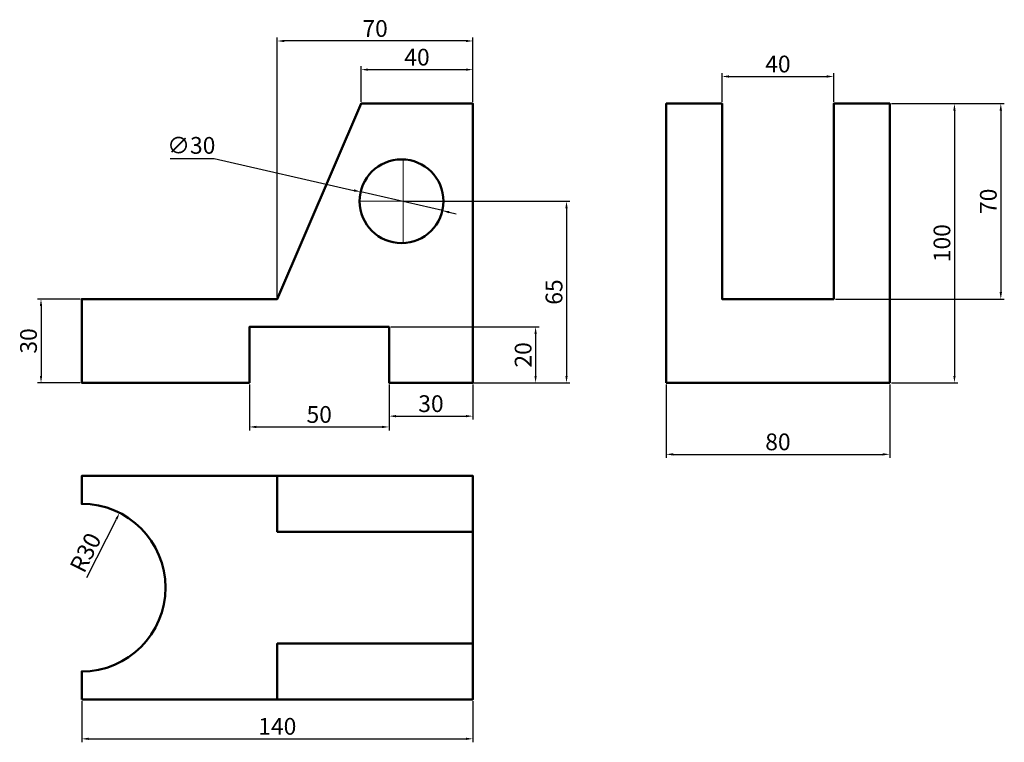
# Model space of a CAD drawing. Units: millimetres. Extents: x 2 to 354, y 5 to 263.
import ezdxf

# ---------------------------------------------------------------- set-up
doc = ezdxf.new("R2010")
doc.units = ezdxf.units.MM
doc.linetypes.add('CENTER', pattern=[50.8, 31.75, -6.35, 6.35, -6.35])
for name, color, linetype, lineweight in [('M-CNTR', 1, 'CENTER', 18), ('M-DIMS', 2, 'Continuous', 25), ('M-OUTL', 7, 'Continuous', 50)]:
    doc.layers.add(name, color=color, linetype=linetype, lineweight=lineweight)
doc.styles.get("Standard").update_dxf_attribs({"font": 'arial.ttf'})
doc.dimstyles.new('ISO-25', dxfattribs={"dimtxt": 6, "dimasz": 2.5, "dimexe": 1.25, "dimexo": 0.625, "dimtad": 1, "dimtoh": 1, "dimdec": 0, "dimtxsty": 'Standard', "dimcen": 2.5, "dimadec": 0, "dimazin": 0, "dimtfac": 1, "dimtdec": 0, "dimtmove": 0, "dimatfit": 3, "dimfxl": 1, "dimarcsym": 0})

# ---------------------------------------------------------------- blocks, each defined once
blk = doc.blocks.new('*D1')
at = {"layer": 'Defpoints', "color": 0, "transparency": 16777216}
for p in [(93.8, 255.73), (163.8, 233.33), (93.8, 163.33)]:
    blk.add_point(p, dxfattribs=at)
at = {"layer": 'M-DIMS', "color": 0, "lineweight": -2, "transparency": 16777216}
for p, q in [((93.8, 163.96), (93.8, 256.98)), ((161.3, 255.73), (96.3, 255.73)), ((163.8, 233.96), (163.8, 256.98))]:
    blk.add_line(p, q, dxfattribs=at)
at = {"layer": 'M-DIMS', "color": 0, "transparency": 16777216}
for points in [[(96.3, 256.14), (96.3, 255.31), (93.8, 255.73)], [(161.3, 256.14), (161.3, 255.31), (163.8, 255.73)]]:
    blk.add_solid(points, dxfattribs=at)
at = {"layer": 'M-DIMS', "color": 0, "transparency": 16777216, "insert": (128.8, 259.42), "char_height": 6, "attachment_point": 5}
blk.add_mtext('70', dxfattribs=at)
blk = doc.blocks.new('*D2')
at = {"layer": 'Defpoints', "color": 0, "transparency": 16777216}
for p in [(163.8, 245.47), (123.8, 233.33), (163.8, 233.33)]:
    blk.add_point(p, dxfattribs=at)
at = {"layer": 'M-DIMS', "color": 0, "lineweight": -2, "transparency": 16777216}
for p, q in [((123.8, 233.96), (123.8, 246.72)), ((163.8, 233.96), (163.8, 246.72)), ((126.3, 245.47), (161.3, 245.47))]:
    blk.add_line(p, q, dxfattribs=at)
at = {"layer": 'M-DIMS', "color": 0, "transparency": 16777216}
for points in [[(126.3, 245.88), (126.3, 245.05), (123.8, 245.47)], [(161.3, 245.88), (161.3, 245.05), (163.8, 245.47)]]:
    blk.add_solid(points, dxfattribs=at)
at = {"layer": 'M-DIMS', "color": 0, "transparency": 16777216, "insert": (143.8, 249.16), "char_height": 6, "attachment_point": 5}
blk.add_mtext('40', dxfattribs=at)
blk = doc.blocks.new('*D3')
at = {"layer": 'Defpoints', "color": 0, "transparency": 16777216}
for p in [(133.8, 153.33), (133.8, 133.33), (186.25, 133.33)]:
    blk.add_point(p, dxfattribs=at)
at = {"layer": 'M-DIMS', "color": 0, "lineweight": -2, "transparency": 16777216}
for p, q in [((134.43, 153.33), (187.5, 153.33)), ((186.25, 150.83), (186.25, 135.83)), ((134.43, 133.33), (187.5, 133.33))]:
    blk.add_line(p, q, dxfattribs=at)
at = {"layer": 'M-DIMS', "color": 0, "transparency": 16777216}
for points in [[(185.84, 150.83), (186.67, 150.83), (186.25, 153.33)], [(185.84, 135.83), (186.67, 135.83), (186.25, 133.33)]]:
    blk.add_solid(points, dxfattribs=at)
at = {"layer": 'M-DIMS', "color": 0, "transparency": 16777216, "insert": (182.57, 143.33), "char_height": 6, "attachment_point": 5, "rotation": 90}
blk.add_mtext('20', dxfattribs=at)
blk = doc.blocks.new('*D4')
at = {"layer": 'Defpoints', "color": 0, "transparency": 16777216}
for p in [(138.8, 198.33), (133.8, 133.33), (197.32, 133.33)]:
    blk.add_point(p, dxfattribs=at)
at = {"layer": 'M-DIMS', "color": 0, "lineweight": -2, "transparency": 16777216}
for p, q in [((139.43, 198.33), (198.57, 198.33)), ((197.32, 195.83), (197.32, 135.83)), ((134.43, 133.33), (198.57, 133.33))]:
    blk.add_line(p, q, dxfattribs=at)
at = {"layer": 'M-DIMS', "color": 0, "transparency": 16777216}
for points in [[(196.9, 195.83), (197.74, 195.83), (197.32, 198.33)], [(196.9, 135.83), (197.74, 135.83), (197.32, 133.33)]]:
    blk.add_solid(points, dxfattribs=at)
at = {"layer": 'M-DIMS', "color": 0, "transparency": 16777216, "insert": (193.63, 165.83), "char_height": 6, "attachment_point": 5, "rotation": 90}
blk.add_mtext('65', dxfattribs=at)
blk = doc.blocks.new('*D5')
at = {"layer": 'Defpoints', "color": 0, "transparency": 16777216}
for p in [(123.66, 201.68), (152.9, 194.98)]:
    blk.add_point(p, dxfattribs=at)
at = {"layer": 'M-DIMS', "color": 0, "lineweight": -2, "transparency": 16777216}
for p, q in [((55.45, 213.71), (71.18, 213.71)), ((71.18, 213.71), (121.22, 202.24)), ((152.9, 194.98), (123.66, 201.68)), ((155.34, 194.42), (157.77, 193.86))]:
    blk.add_line(p, q, dxfattribs=at)
at = {"layer": 'M-DIMS', "color": 0, "transparency": 16777216}
for points in [[(121.31, 202.65), (121.13, 201.84), (123.66, 201.68)], [(155.43, 194.83), (155.24, 194.02), (152.9, 194.98)]]:
    blk.add_solid(points, dxfattribs=at)
at = {"layer": 'M-DIMS', "color": 0, "transparency": 16777216, "insert": (63, 217.57), "char_height": 6, "attachment_point": 5}
blk.add_mtext('∅30', dxfattribs=at)
blk = doc.blocks.new('*D6')
at = {"layer": 'Defpoints', "color": 0, "transparency": 16777216}
for p in [(23.8, 163.33), (9.22, 133.33), (23.8, 133.33)]:
    blk.add_point(p, dxfattribs=at)
at = {"layer": 'M-DIMS', "color": 0, "lineweight": -2, "transparency": 16777216}
for p, q in [((23.18, 163.33), (7.97, 163.33)), ((9.22, 160.83), (9.22, 135.83)), ((23.18, 133.33), (7.97, 133.33))]:
    blk.add_line(p, q, dxfattribs=at)
at = {"layer": 'M-DIMS', "color": 0, "transparency": 16777216}
for points in [[(8.8, 160.83), (9.63, 160.83), (9.22, 163.33)], [(8.8, 135.83), (9.63, 135.83), (9.22, 133.33)]]:
    blk.add_solid(points, dxfattribs=at)
at = {"layer": 'M-DIMS', "color": 0, "transparency": 16777216, "insert": (5.52, 148.33), "char_height": 6, "attachment_point": 5, "rotation": 90}
blk.add_mtext('30', dxfattribs=at)
blk = doc.blocks.new('*D7')
at = {"layer": 'Defpoints', "color": 0, "transparency": 16777216}
for p in [(83.8, 133.33), (133.8, 133.33), (133.8, 117.53)]:
    blk.add_point(p, dxfattribs=at)
at = {"layer": 'M-DIMS', "color": 0, "lineweight": -2, "transparency": 16777216}
for p, q in [((83.8, 132.71), (83.8, 116.28)), ((133.8, 132.71), (133.8, 116.28)), ((86.3, 117.53), (131.3, 117.53))]:
    blk.add_line(p, q, dxfattribs=at)
at = {"layer": 'M-DIMS', "color": 0, "transparency": 16777216}
for points in [[(86.3, 117.95), (86.3, 117.11), (83.8, 117.53)], [(131.3, 117.95), (131.3, 117.11), (133.8, 117.53)]]:
    blk.add_solid(points, dxfattribs=at)
at = {"layer": 'M-DIMS', "color": 0, "transparency": 16777216, "insert": (108.8, 121.22), "char_height": 6, "attachment_point": 5}
blk.add_mtext('50', dxfattribs=at)
blk = doc.blocks.new('*D8')
at = {"layer": 'Defpoints', "color": 0, "transparency": 16777216}
for p in [(133.8, 133.33), (163.8, 133.33), (163.8, 121.4)]:
    blk.add_point(p, dxfattribs=at)
at = {"layer": 'M-DIMS', "color": 0, "lineweight": -2, "transparency": 16777216}
for p, q in [((133.8, 132.71), (133.8, 120.15)), ((163.8, 132.71), (163.8, 120.15)), ((136.3, 121.4), (161.3, 121.4))]:
    blk.add_line(p, q, dxfattribs=at)
at = {"layer": 'M-DIMS', "color": 0, "transparency": 16777216}
for points in [[(136.3, 121.81), (136.3, 120.98), (133.8, 121.4)], [(161.3, 121.81), (161.3, 120.98), (163.8, 121.4)]]:
    blk.add_solid(points, dxfattribs=at)
at = {"layer": 'M-DIMS', "color": 0, "transparency": 16777216, "insert": (148.8, 125.09), "char_height": 6, "attachment_point": 5}
blk.add_mtext('30', dxfattribs=at)
blk = doc.blocks.new('*D9')
at = {"layer": 'Defpoints', "color": 0, "transparency": 16777216}
for p in [(37.33, 86.77), (23.8, 59.99)]:
    blk.add_point(p, dxfattribs=at)
at = {"layer": 'M-DIMS', "color": 0, "lineweight": -2, "transparency": 16777216}
blk.add_line((25.62, 63.59), (36.2, 84.54), dxfattribs=at)
at = {"layer": 'M-DIMS', "color": 0, "transparency": 16777216}
blk.add_solid([(35.83, 84.72), (36.57, 84.35), (37.33, 86.77)], dxfattribs=at)
at = {"layer": 'M-DIMS', "color": 0, "transparency": 16777216, "insert": (25.84, 72.2), "char_height": 6, "attachment_point": 5, "rotation": 63.2046}
blk.add_mtext('R30', dxfattribs=at)
blk = doc.blocks.new('*D10')
at = {"layer": 'Defpoints', "color": 0, "transparency": 16777216}
for p in [(23.8, 19.99), (163.8, 19.99), (163.8, 5.86)]:
    blk.add_point(p, dxfattribs=at)
at = {"layer": 'M-DIMS', "color": 0, "lineweight": -2, "transparency": 16777216}
for p, q in [((23.8, 19.36), (23.8, 4.61)), ((163.8, 19.36), (163.8, 4.61)), ((26.3, 5.86), (161.3, 5.86))]:
    blk.add_line(p, q, dxfattribs=at)
at = {"layer": 'M-DIMS', "color": 0, "transparency": 16777216}
for points in [[(26.3, 6.28), (26.3, 5.45), (23.8, 5.86)], [(161.3, 6.28), (161.3, 5.45), (163.8, 5.86)]]:
    blk.add_solid(points, dxfattribs=at)
at = {"layer": 'M-DIMS', "color": 0, "transparency": 16777216, "insert": (93.8, 9.55), "char_height": 6, "attachment_point": 5}
blk.add_mtext('140', dxfattribs=at)
blk = doc.blocks.new('*D11')
at = {"layer": 'Defpoints', "color": 0, "transparency": 16777216}
for p in [(293, 243.01), (253, 233.33), (293, 233.33)]:
    blk.add_point(p, dxfattribs=at)
at = {"layer": 'M-DIMS', "color": 0, "lineweight": -2, "transparency": 16777216}
for p, q in [((253, 233.96), (253, 244.26)), ((293, 233.96), (293, 244.26)), ((255.5, 243.01), (290.5, 243.01))]:
    blk.add_line(p, q, dxfattribs=at)
at = {"layer": 'M-DIMS', "color": 0, "transparency": 16777216}
for points in [[(255.5, 243.43), (255.5, 242.6), (253, 243.01)], [(290.5, 243.43), (290.5, 242.6), (293, 243.01)]]:
    blk.add_solid(points, dxfattribs=at)
at = {"layer": 'M-DIMS', "color": 0, "transparency": 16777216, "insert": (273, 246.7), "char_height": 6, "attachment_point": 5}
blk.add_mtext('40', dxfattribs=at)
blk = doc.blocks.new('*D12')
at = {"layer": 'Defpoints', "color": 0, "transparency": 16777216}
for p in [(313, 233.33), (293, 163.33), (352.78, 163.33)]:
    blk.add_point(p, dxfattribs=at)
at = {"layer": 'M-DIMS', "color": 0, "lineweight": -2, "transparency": 16777216}
for p, q in [((313.63, 233.33), (354.03, 233.33)), ((352.78, 230.83), (352.78, 165.83)), ((293.63, 163.33), (354.03, 163.33))]:
    blk.add_line(p, q, dxfattribs=at)
at = {"layer": 'M-DIMS', "color": 0, "transparency": 16777216}
for points in [[(352.36, 230.83), (353.2, 230.83), (352.78, 233.33)], [(352.36, 165.83), (353.2, 165.83), (352.78, 163.33)]]:
    blk.add_solid(points, dxfattribs=at)
at = {"layer": 'M-DIMS', "color": 0, "transparency": 16777216, "insert": (349.09, 198.33), "char_height": 6, "attachment_point": 5, "rotation": 90}
blk.add_mtext('70', dxfattribs=at)
blk = doc.blocks.new('*D13')
at = {"layer": 'Defpoints', "color": 0, "transparency": 16777216}
for p in [(313, 233.33), (313, 133.33), (336.18, 133.33)]:
    blk.add_point(p, dxfattribs=at)
at = {"layer": 'M-DIMS', "color": 0, "lineweight": -2, "transparency": 16777216}
for p, q in [((313.63, 233.33), (337.43, 233.33)), ((336.18, 230.83), (336.18, 135.83)), ((313.63, 133.33), (337.43, 133.33))]:
    blk.add_line(p, q, dxfattribs=at)
at = {"layer": 'M-DIMS', "color": 0, "transparency": 16777216}
for points in [[(335.77, 230.83), (336.6, 230.83), (336.18, 233.33)], [(335.77, 135.83), (336.6, 135.83), (336.18, 133.33)]]:
    blk.add_solid(points, dxfattribs=at)
at = {"layer": 'M-DIMS', "color": 0, "transparency": 16777216, "insert": (332.49, 183.33), "char_height": 6, "attachment_point": 5, "rotation": 90}
blk.add_mtext('100', dxfattribs=at)
blk = doc.blocks.new('*D14')
at = {"layer": 'Defpoints', "color": 0, "transparency": 16777216}
for p in [(233, 133.33), (313, 133.33), (313, 107.72)]:
    blk.add_point(p, dxfattribs=at)
at = {"layer": 'M-DIMS', "color": 0, "lineweight": -2, "transparency": 16777216}
for p, q in [((233, 132.71), (233, 106.47)), ((313, 132.71), (313, 106.47)), ((235.5, 107.72), (310.5, 107.72))]:
    blk.add_line(p, q, dxfattribs=at)
at = {"layer": 'M-DIMS', "color": 0, "transparency": 16777216}
for points in [[(235.5, 108.14), (235.5, 107.3), (233, 107.72)], [(310.5, 108.14), (310.5, 107.3), (313, 107.72)]]:
    blk.add_solid(points, dxfattribs=at)
at = {"layer": 'M-DIMS', "color": 0, "transparency": 16777216, "insert": (273, 111.41), "char_height": 6, "attachment_point": 5}
blk.add_mtext('80', dxfattribs=at)

msp = doc.modelspace()

# ---------------------------------------------------------------- linework, layer by layer
at = {"layer": 'M-CNTR'}
for p, q in [((138.8, 183.34), (138.8, 213.32)), ((123.28, 198.33), (153.28, 198.33))]:
    msp.add_line(p, q, dxfattribs=at)
at = {"layer": 'M-OUTL'}
for points in [[(83.8, 133.33), (83.8, 153.33), (133.8, 153.33), (133.8, 133.33), (163.8, 133.33), (163.8, 233.33), (123.8, 233.33), (93.8, 163.33), (23.8, 163.33), (23.8, 133.33)], [(233, 133.33), (233, 233.33), (253, 233.33), (253, 163.33), (293, 163.33), (293, 233.33), (313, 233.33), (313, 133.33)]]:
    msp.add_lwpolyline(points, close=True, dxfattribs=at)
msp.add_lwpolyline([(23.8, 19.99), (23.8, 29.99, 1), (23.8, 89.99), (23.8, 99.99), (163.8, 99.99), (163.8, 19.99)], format="xyb", close=True, dxfattribs=at)
for points in [[(163.8, 79.99), (93.8, 79.99), (93.8, 99.99)], [(93.8, 19.99), (93.8, 39.99), (163.8, 39.99)]]:
    msp.add_lwpolyline(points, dxfattribs=at)
msp.add_circle((138.28, 198.33), 15, dxfattribs=at)

# ---------------------------------------------------------------- dimensions: what is measured, and where the dimension line sits
at = {"layer": 'M-DIMS'}
for base, p1, p2, picture, middle in [((93.8, 255.73), (163.8, 233.33), (93.8, 163.33), '*D1', (128.8, 259.42)), ((163.8, 245.47), (123.8, 233.33), (163.8, 233.33), '*D2', (143.8, 249.16)), ((293, 243.01), (253, 233.33), (293, 233.33), '*D11', (273, 246.7)), ((133.8, 117.53), (83.8, 133.33), (133.8, 133.33), '*D7', (108.8, 121.22)), ((163.8, 121.4), (133.8, 133.33), (163.8, 133.33), '*D8', (148.8, 125.09)), ((313, 107.72), (233, 133.33), (313, 133.33), '*D14', (273, 111.41)), ((163.8, 5.86), (23.8, 19.99), (163.8, 19.99), '*D10', (93.8, 9.55))]:
    dim = msp.add_linear_dim(base=base, p1=p1, p2=p2, dimstyle='ISO-25', override={"dimclrd": 0, "dimclre": 0, "dimclrt": 0}, dxfattribs=at)
    dim.commit()
    dim.dimension.update_dxf_attribs({"geometry": picture, "text_midpoint": middle})
for base, p1, p2, picture, middle in [((352.78, 163.33), (313, 233.33), (293, 163.33), '*D12', (349.09, 198.33)), ((336.18, 133.33), (313, 233.33), (313, 133.33), '*D13', (332.49, 183.33)), ((197.32, 133.33), (138.8, 198.33), (133.8, 133.33), '*D4', (193.63, 165.83)), ((9.22, 133.33), (23.8, 163.33), (23.8, 133.33), '*D6', (5.52, 148.33)), ((186.25, 133.33), (133.8, 153.33), (133.8, 133.33), '*D3', (182.57, 143.33))]:
    dim = msp.add_linear_dim(base=base, p1=p1, p2=p2, angle=90, dimstyle='ISO-25', override={"dimclrd": 0, "dimclre": 0, "dimclrt": 0}, dxfattribs=at)
    dim.commit()
    dim.dimension.update_dxf_attribs({"geometry": picture, "text_midpoint": middle})
dim = msp.add_diameter_dim_2p(p1=(152.9, 194.98), p2=(123.66, 201.68), dimstyle='ISO-25', override={"dimclrd": 0, "dimclre": 0, "dimclrt": 0}, dxfattribs=at)
dim.commit()
dim.dimension.update_dxf_attribs({"geometry": '*D5', "text_midpoint": (71.18, 213.71), "dimtype": 163})
dim = msp.add_radius_dim(center=(23.8, 59.99), mpoint=(37.33, 86.77), dimstyle='ISO-25', override={"dimclrd": 0, "dimclre": 0, "dimclrt": 0}, dxfattribs=at)
dim.commit()
dim.dimension.update_dxf_attribs({"geometry": '*D9', "text_midpoint": (29.13, 70.54), "dimtype": 164})

doc.saveas('drawing.dxf')
